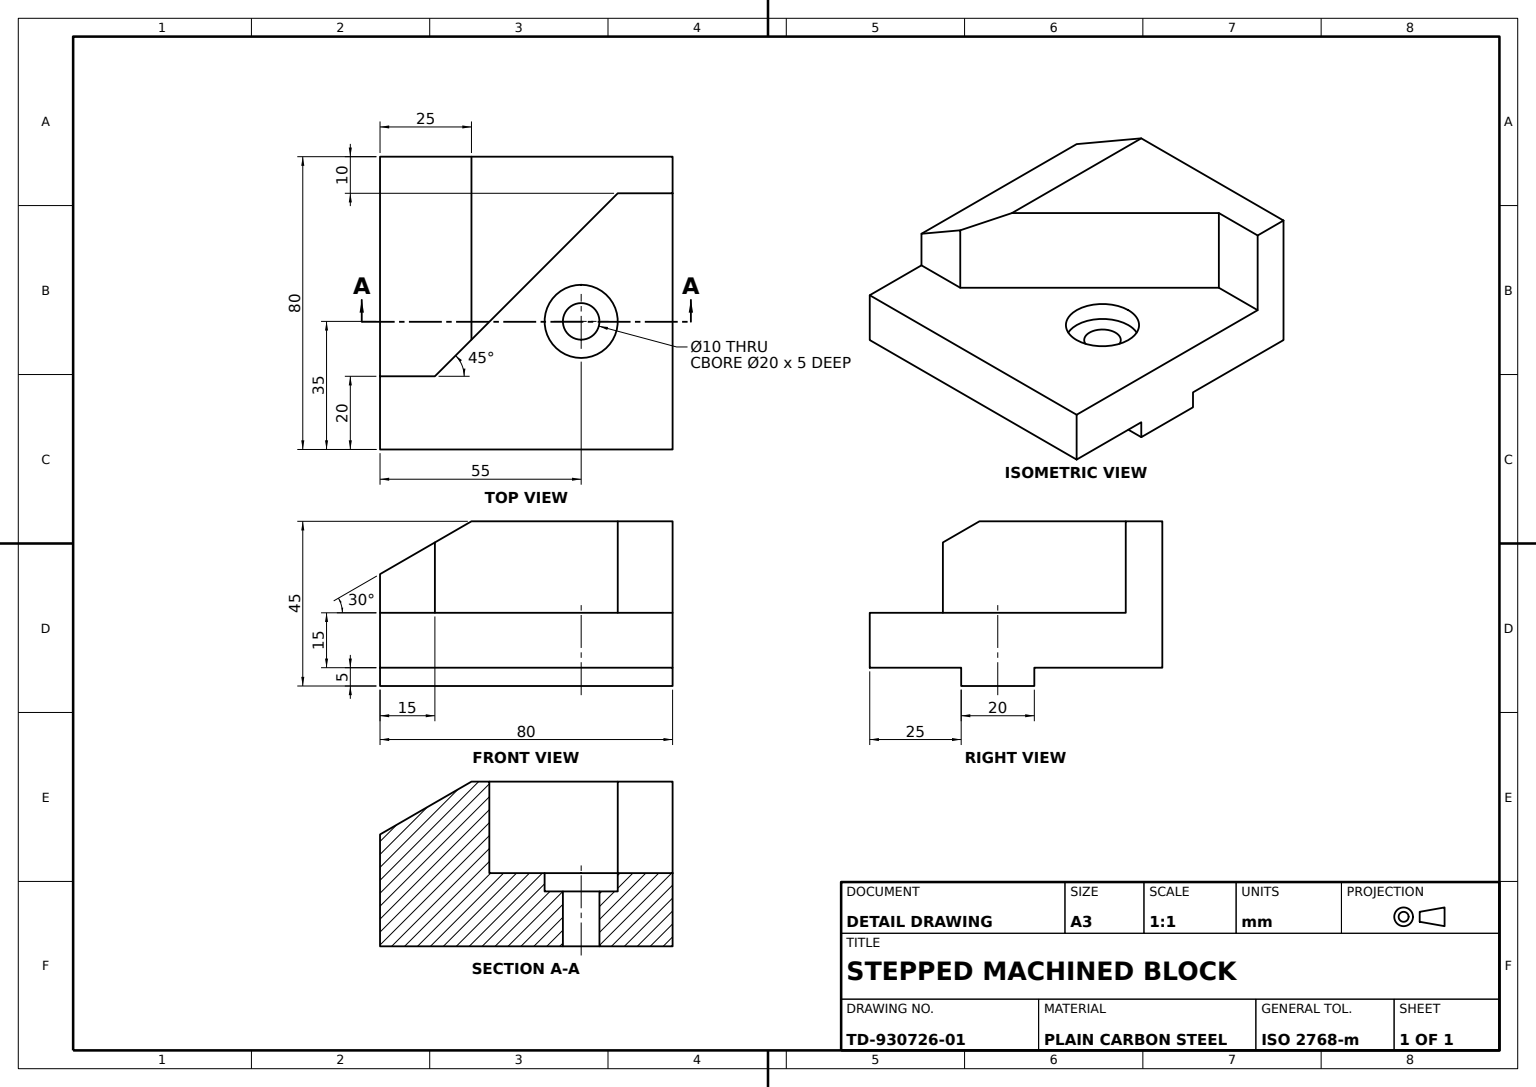
from build123d import *

# Parameters (mm, degrees)
BASE_PLATE_SKETCH_80X80_W          = 80
BASE_PLATE_SKETCH_80X80_H          = 80
BASE_PLATE_80X80X15_DEPTH          = 15
LOCATING_KEY_SKETCH_20X25_W        = 80
LOCATING_KEY_SKETCH_20X25_H        = 20
LOCATING_KEY_20X25X5_DEPTH         = 5
MOUNTING_HOLE_SKETCH_10_R          = 5
MOUNTING_HOLE_10_DEPTH             = 60
COUNTERBORE_SKETCH_20_R            = 10
COUNTERBORE_20X5_DEPTH             = 5
STOP_BLOCK_25_HIGH_DEPTH           = 25
V_STOP_ANGLED_FACE_CUT_30DEG_DEPTH = 100


with BuildPart() as part:
    # Base Plate Sketch 80x80 → Base Plate 80x80x15 (new body)
    with BuildSketch(Plane(origin=(0, 0, 0), x_dir=(1, 0, 0), z_dir=(0, 1, 0))):
        Rectangle(BASE_PLATE_SKETCH_80X80_W, BASE_PLATE_SKETCH_80X80_H)
    extrude(amount=BASE_PLATE_80X80X15_DEPTH)

    # Locating Key Sketch 20x25 → Locating Key 20x25x5 (add)
    with BuildSketch(Plane.XZ):
        with Locations((0, 5)):
            Rectangle(LOCATING_KEY_SKETCH_20X25_W, LOCATING_KEY_SKETCH_20X25_H)
    extrude(amount=LOCATING_KEY_20X25X5_DEPTH)

    # Mounting Hole Sketch Ø10 → Mounting Hole Ø10 (cut)
    with BuildSketch(Plane(origin=(0, 15, 0), x_dir=(1, 0, 0), z_dir=(0, 1, 0))):
        with Locations(Location((15, -5, 0), (0, 0, 270))):
            Circle(MOUNTING_HOLE_SKETCH_10_R)
    extrude(amount=-MOUNTING_HOLE_10_DEPTH, mode=Mode.SUBTRACT)

    # Counterbore Sketch Ø20 → Counterbore Ø20x5 (cut)
    with BuildSketch(Plane(origin=(0, 15, 0), x_dir=(1, 0, 0), z_dir=(0, 1, 0))):
        with Locations(Location((15, -5, 0), (0, 0, 270))):
            Circle(COUNTERBORE_SKETCH_20_R)
    extrude(amount=-COUNTERBORE_20X5_DEPTH, mode=Mode.SUBTRACT)

    # Stop Block Profile Sketch → Stop Block 25 High (add)
    with BuildSketch(Plane(origin=(0, 15, 0), x_dir=(1, 0, 0), z_dir=(0, 1, 0))):
        Polygon((40, 40), (40, 30), (25, 30), (-25, -20), (-40, -20), (-40, 40), align=None)
    extrude(amount=STOP_BLOCK_25_HIGH_DEPTH)

    # V-Stop Angle Sketch 30deg → V-Stop Angled Face Cut 30deg (cut)
    with BuildSketch(Plane(origin=(0, 0, -40), x_dir=(-1, 0, 0), z_dir=(0, 0, -1))):
        Polygon((40, 25.56624327), (15, 40), (40, 40), align=None)
    extrude(amount=-V_STOP_ANGLED_FACE_CUT_30DEG_DEPTH, mode=Mode.SUBTRACT)


solid = part.part
